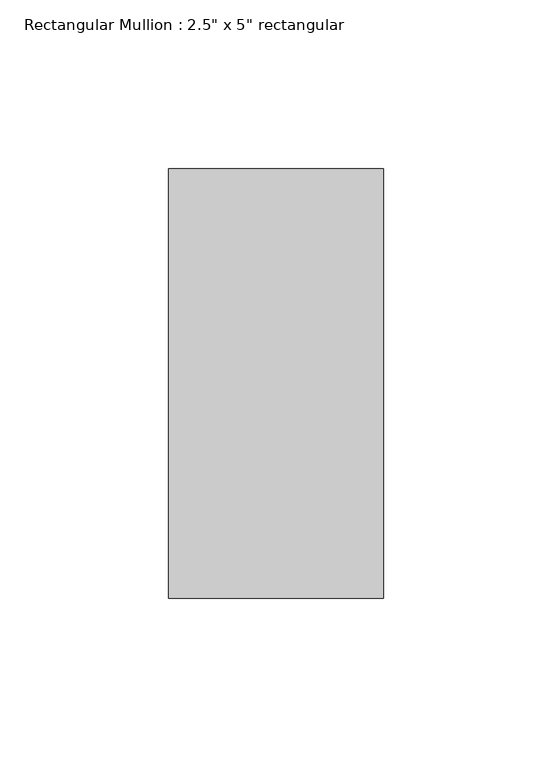
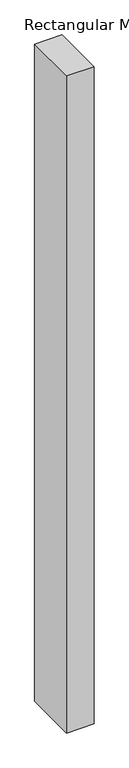
"""IFC4 building model written with IfcOpenShell, lengths in millimetres: member geometry."""

from ifc_helpers import new_model, si_unit, frame, origin, place, context, project, spatial, polyline, outline, extrude, source, transform, mapped, element, save


def member_5210a67a(model_context):
    return source(origin(), model_context, "Body", "SweptSolid", [
        extrude(outline(polyline([(31.75, 63.5), (31.75, -63.5), (-31.75, -63.5), (-31.75, 63.5), (31.75, 63.5)])), frame((0.0, 0.0, -1600.1465467), z_axis=(0.0, 0.0, 1.0), x_axis=(1.0, 0.0, 0.0)), (0.0, 0.0, 1.0), 1600.1465467),
    ])


if __name__ == "__main__":
    model = new_model("IFC4")
    model_context = context("Model", 3, world=origin())
    ifc_project = project(units=[si_unit("LENGTHUNIT", "METRE", prefix="MILLI")], contexts=[model_context])
    site = spatial("IfcSite", under=ifc_project)
    building = spatial("IfcBuilding", under=site)
    placement = place(None, origin())
    member_shape = member_5210a67a(model_context)
    element("IfcMember", 1, ObjectType="Rectangular Mullion : 2.5\" x 5\" rectangular", at=placement, inside=building, context=model_context, shape_type="MappedRepresentation", body=[
        mapped(member_shape, transform((0.0, 0.0, 0.0), x_axis=(1.0, 0.0, 0.0), y_axis=(0.0, 1.0, 0.0), z_axis=(0.0, 0.0, 1.0))),
    ])
    save(model, "model.ifc")

# Revit data of these elements
# Type "Rectangular Mullion : 2.5\" x 5\" rectangular"
#   built-in parameter 1007304 = 0.416667 (stored number, unit not read)
#   built-in parameter 1007301 = 0.104167 (stored number, unit not read)
#   built-in parameter 1007300 = 0.104167 (stored number, unit not read)
# Element 1 (IfcMember, "Rectangular Mullion : 2.5\" x 5\" rectangular")
#   Materials on its faces: "Aluminum"
# Materials
#   "Aluminum": class "Metal", colour RGB 247 247 247, transparency 0, Description = "Aluminum 6061", Cost = 0
